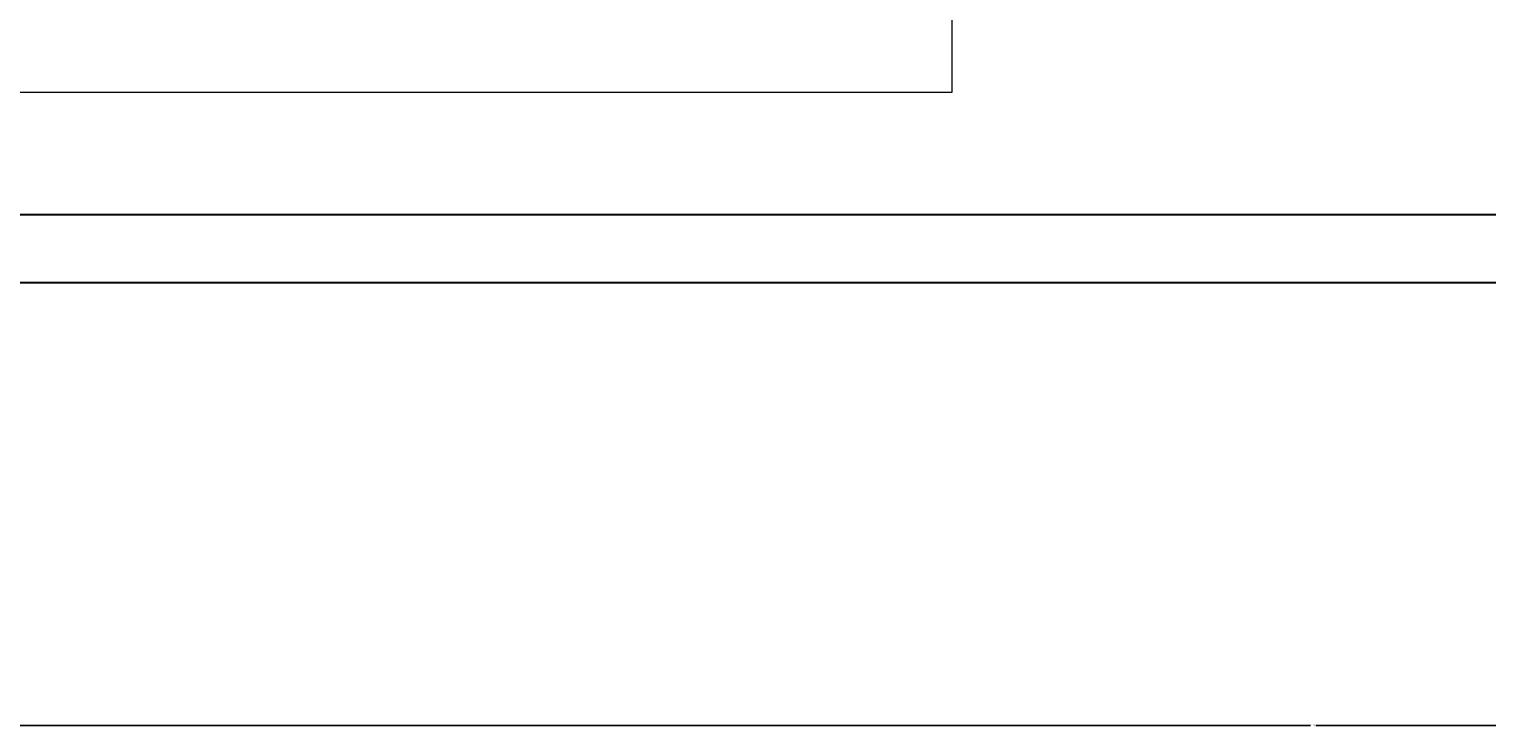
# Model space of a CAD drawing. Units: inches. Extents: x -46 to 1145, y -527 to 760.
# Tile 5 of 57: x 380 to 573, y -527 to -435. Entities that reach past the tile are written whole.
import ezdxf

# ---------------------------------------------------------------- set-up
doc = ezdxf.new("R2010")
doc.units = ezdxf.units.IN
doc.header["$MEASUREMENT"] = 0
for name, color, linetype, lineweight in [('A-ANNO-DIMS', 2, 'Continuous', 18), ('C-PKNG', 8, 'Continuous', 18), ('C-SITE', 7, 'Continuous', 30)]:
    doc.layers.add(name, color=color, linetype=linetype, lineweight=lineweight)
doc.styles.get("Standard").update_dxf_attribs({"font": 'arial.ttf'})
doc.dimstyles.get("Standard").update_dxf_attribs({"dimtxt": 0.18, "dimasz": 0.18, "dimexe": 0.18, "dimexo": 0.0625, "dimgap": 0.09, "dimtad": 0, "dimtih": 1, "dimtoh": 1, "dimdec": 0, "dimzin": 0, "dimdsep": 46, "dimlunit": 3, "dimtxsty": 'Standard', "dimcen": 0.09, "dimadec": 0, "dimazin": 0, "dimtfac": 1, "dimtdec": 0, "dimtofl": 0, "dimtmove": 0, "dimatfit": 3, "dimfxl": 1, "dimtolj": 1, "dimtzin": 0, "dimarcsym": 0})

# ---------------------------------------------------------------- blocks, each defined once
blk = doc.blocks.new('*D684')
at = {"layer": 'A-ANNO-DIMS', "color": 0, "lineweight": -2, "transparency": 16777216}
for p, q in [((12.56, -468.54), (12.56, -527.26)), ((1086.56, -468.54), (1086.56, -527.26)), ((12.74, -527.08), (549.21, -527.08)), ((1086.38, -527.08), (549.91, -527.08))]:
    blk.add_line(p, q, dxfattribs=at)
at = {"layer": 'A-ANNO-DIMS', "color": 0, "transparency": 16777216}
for points in [[(12.74, -527.05), (12.74, -527.11), (12.56, -527.08)], [(1086.38, -527.05), (1086.38, -527.11), (1086.56, -527.08)]]:
    blk.add_solid(points, dxfattribs=at)
at = {"layer": 'Defpoints', "color": 0, "transparency": 16777216}
for p in [(12.56, -468.48), (1086.56, -468.48), (1086.56, -527.08)]:
    blk.add_point(p, dxfattribs=at)
at = {"layer": 'A-ANNO-DIMS', "color": 0, "transparency": 16777216, "insert": (549.56, -527.08), "char_height": 0.18, "attachment_point": 5}
blk.add_mtext('\\A1;1074', dxfattribs=at)
blk = doc.blocks.new('*D702')
at = {"layer": 'A-ANNO-DIMS', "color": 0, "lineweight": -2, "transparency": 16777216}
for p, q in [((189.63, -39.48), (1145.34, -39.48)), ((1145.16, -39.66), (1145.16, -249.3)), ((1145.16, -459.3), (1145.16, -249.66)), ((183.63, -459.48), (1145.34, -459.48))]:
    blk.add_line(p, q, dxfattribs=at)
at = {"layer": 'A-ANNO-DIMS', "color": 0, "transparency": 16777216}
for points in [[(1145.13, -39.66), (1145.19, -39.66), (1145.16, -39.48)], [(1145.13, -459.3), (1145.19, -459.3), (1145.16, -459.48)]]:
    blk.add_solid(points, dxfattribs=at)
at = {"layer": 'Defpoints', "color": 0, "transparency": 16777216}
for p in [(189.56, -39.48), (1145.16, -39.48), (183.56, -459.48)]:
    blk.add_point(p, dxfattribs=at)
at = {"layer": 'A-ANNO-DIMS', "color": 0, "transparency": 16777216, "insert": (1145.16, -249.48), "char_height": 0.18, "attachment_point": 5}
blk.add_mtext('\\A1;420', dxfattribs=at)

msp = doc.modelspace()

# ---------------------------------------------------------------- linework, layer by layer
at = {"layer": 'C-PKNG'}
msp.add_lwpolyline([(501.7297, -443.2988), (273.5156, -443.2988), (273.5156, -345.0009), (501.7297, -345.0009)], close=True, dxfattribs=at)
at = {"layer": 'C-SITE'}
for p, q in [((21.5637, -459.4824), (1077.5637, -459.4824)), ((12.5637, -468.4824), (1086.5637, -468.4824))]:
    msp.add_line(p, q, dxfattribs=at)

# ---------------------------------------------------------------- dimensions: what is measured, and where the dimension line sits
at = {"layer": 'A-ANNO-DIMS'}
dim = msp.add_linear_dim(base=(1145.1637, -39.4824), p1=(183.5637, -459.4824), p2=(189.5637, -39.4824), angle=90, dimstyle='Standard', override={"dimdec": 0, "dimlfac": 1, "dimrnd": 0, "dimzin": 0, "dimdsep": 46, "dimlunit": 2}, dxfattribs=at)
dim.commit()
dim.dimension.update_dxf_attribs({"geometry": '*D702', "text_midpoint": (1145.1637, -249.4824)})
dim = msp.add_linear_dim(base=(1086.5637, -527.0824), p1=(12.5637, -468.4824), p2=(1086.5637, -468.4824), dimstyle='Standard', override={"dimdec": 0, "dimlfac": 1, "dimrnd": 0, "dimzin": 0, "dimdsep": 46, "dimlunit": 2}, dxfattribs=at)
dim.commit()
dim.dimension.update_dxf_attribs({"geometry": '*D684', "text_midpoint": (549.5637, -527.0824)})

doc.saveas('drawing.dxf')
